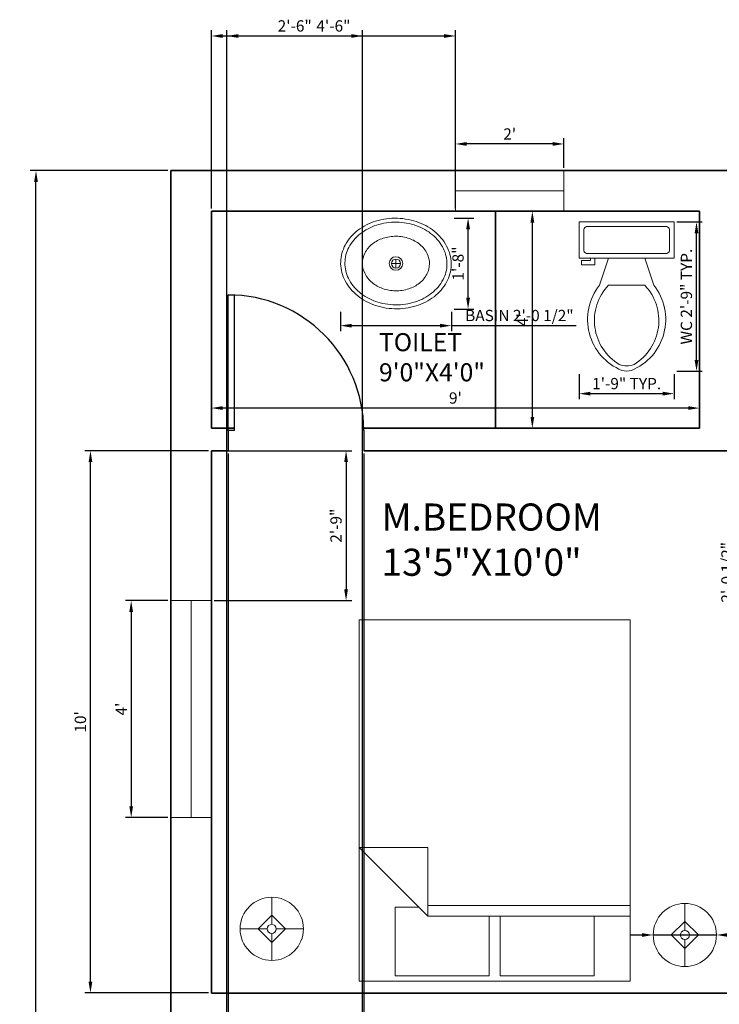
# Model space of a CAD drawing. Units: inches. Extents: x 3889 to 4254, y 3310 to 3958.
# Tile 5 of 6: x 3891 to 4046, y 3738 to 3956. Entities that reach past the tile are written whole.
import ezdxf

# ---------------------------------------------------------------- set-up
doc = ezdxf.new("R2010")
doc.units = ezdxf.units.IN
for name, color, linetype, lineweight in [('A-AREA-IDEN', 11, 'Continuous', 18), ('A-FLOR-FIXT', 130, 'Continuous', 18), ('A-WALL', 7, 'Continuous', 35), ('DIM', 81, 'Continuous', 18), ('DOOR', 1, 'Continuous', 25), ('FURNITURES', 130, 'Continuous', 18), ('WINDOW', 3, 'Continuous', 18)]:
    doc.layers.add(name, color=color, linetype=linetype, lineweight=lineweight)
doc.styles.get("Standard").update_dxf_attribs({"font": 'arial.ttf'})
doc.dimstyles.new('ISO-25', dxfattribs={"dimtxt": 2.5, "dimasz": 2.5, "dimexe": 1.25, "dimexo": 0.625, "dimtad": 1, "dimlunit": 3, "dimtxsty": 'Standard', "dimcen": 2.5, "dimadec": 0, "dimazin": 0, "dimtfac": 1, "dimtmove": 0, "dimatfit": 3, "dimfxl": 1, "dimarcsym": 0})

# ---------------------------------------------------------------- blocks, each defined once
blk = doc.blocks.new('*U4')
for p, q in [((0, 0), (0, -6)), ((40, 0), (40, -6))]:
    blk.add_line(p, q)
blk.add_lwpolyline([(0, 0), (0, 40), (1.75, 40), (1.75, 0)], close=True)
blk.add_arc((0, 0), 40, 0, 90)
blk = doc.blocks.new('Sink - Oval top')
for p, q in [((-1, 0), (1, 0)), ((0, 1), (0, -1))]:
    blk.add_line(p, q)
for points in [[(-12.23, 0.39, 0.117634), (-11.46, -3.36, 0.104469), (-8.88, -6.8, 0.090016), (-5.08, -9.07, 0.08192), (-0.32, -10.02, 0.08192), (4.49, -9.38, 0.090016), (8.42, -7.36, 0.104469), (11.22, -4.09, 0.117634), (12.23, -0.39, 0.117634), (11.46, 3.36, 0.104469), (8.88, 6.8, 0.090016), (5.08, 9.07, 0.08192), (0.32, 10.02, 0.08192), (-4.49, 9.38, 0.090016), (-8.42, 7.36, 0.104469), (-11.22, 4.09, 0.117634)], [(-11.29, 0.16, 0.118622), (-10.52, -3.25, 0.104678), (-8.07, -6.36, 0.089562), (-4.54, -8.37, 0.081185), (-0.13, -9.15, 0.081185), (4.3, -8.49, 0.089562), (7.89, -6.58, 0.104678), (10.42, -3.55, 0.118622), (11.29, -0.16, 0.118622), (10.52, 3.25, 0.104678), (8.07, 6.36, 0.089562), (4.54, 8.37, 0.081185), (0.13, 9.15, 0.081185), (-4.3, 8.49, 0.089562), (-7.89, 6.58, 0.104678), (-10.42, 3.55, 0.118622)], [(-7.42, 0.08, 0.118283), (-6.91, -2.17, 0.104607), (-5.29, -4.21, 0.089718), (-2.97, -5.53, 0.081436), (-0.07, -6.04, 0.081436), (2.84, -5.59, 0.089718), (5.2, -4.33, 0.104607), (6.86, -2.32, 0.118283), (7.42, -0.08, 0.118283), (6.91, 2.17, 0.104607), (5.29, 4.21, 0.089718), (2.97, 5.53, 0.081436), (0.07, 6.04, 0.081436), (-2.84, 5.59, 0.089718), (-5.2, 4.33, 0.104607), (-6.86, 2.32, 0.118283)]]:
    blk.add_lwpolyline(points, format="xyb", close=True)
for radius in [1.5, 1]:
    blk.add_circle((0, 0), radius)
blk = doc.blocks.new('Bed - Queen')
for p, q in [((0, -80.00003), (0, 0)), ((0, 0), (59.99999, 0)), ((59.99999, 0), (59.99999, -80.00003)), ((7.99999, -1.2), (28.79998, -1.2)), ((7.99999, -14.4), (7.99999, -1.2)), ((28.79998, -1.2), (28.79998, -14.4)), ((31.19999, -1.2), (51.99999, -1.2)), ((31.19999, -14.4), (31.19999, -1.2)), ((51.99999, -1.2), (51.99999, -16.4)), ((0, -14.4), (44.8, -14.4)), ((59.99999, -29.6), (44.8, -14.4)), ((44.8, -14.4), (44.8, -29.6)), ((44.8, -16.8), (0, -16.8)), ((51.99999, -16.4), (46.79936, -16.4)), ((44.8, -29.6), (59.99999, -29.6)), ((59.99999, -80.00003), (0, -80.00003))]:
    blk.add_line(p, q)
blk = doc.blocks.new('Lamp - Table')
for p, q in [((0, 7), (0, 1)), ((0, 3), (-3, 0)), ((3, 0), (0, 3)), ((-1, 0), (-7, 0)), ((-3, 0), (0, -3)), ((0, -3), (3, 0)), ((1, 0), (7, 0)), ((0, -1), (0, -7))]:
    blk.add_line(p, q)
for radius in [7, 1]:
    blk.add_circle((0, 0), radius)
blk = doc.blocks.new('Toilet - top')
for p, q in [((9.5, -6), (9.5, -2)), ((-10, -8.5), (-8, -8.5)), ((-10, -9.5), (-10, -8.5)), ((-8, -8.5), (-8, -8)), ((-7, -8), (-7, -9.5)), ((-4, -8), (-6, -14)), ((4, -8), (6, -14)), ((-7, -9.5), (-10, -9.5)), ((4, -14), (-4, -14))]:
    blk.add_line(p, q)
blk.add_lwpolyline([(10.5, -8), (10.5, 0), (-10.5, 0), (-10.5, -8)], close=True)
for points in [[(-9.5, -2), (-9.5, -6)], [(8.5, -1), (-8.5, -1)], [(-8.5, -7), (8.5, -7)]]:
    blk.add_lwpolyline(points)
for centre, radius, start, end in [((-8.62, -1.88), 0.884, 81.8699, 188.1301), ((8.62, -1.88), 0.884, 351.8699, 98.1301), ((-8.62, -6.12), 0.884, 171.8699, 278.1301), ((8.62, -6.12), 0.884, 261.8699, 8.1301), ((3.52, -21.58), 12.17, 141.4691, 247.9714), ((4.2, -21.82), 11.33, 136.3677, 238.9468), ((-3.52, -21.58), 12.17, 292.0284, 38.5307), ((-4.2, -21.82), 11.33, 301.053, 43.6321), ((0, -27.88), 4, 245.7318, 294.2682), ((0, -29), 4, 254.8605, 285.1395)]:
    blk.add_arc(centre, radius, start, end)
blk = doc.blocks.new('*D21')
at = {"layer": 'Defpoints', "color": 0, "transparency": 16777216}
for p in [(3924.84, 3826.95), (3916.1, 3778.95), (3924.84, 3778.95)]:
    blk.add_point(p, dxfattribs=at)
at = {"layer": 'DIM', "color": 0, "lineweight": -2, "transparency": 16777216}
for p, q in [((3924.22, 3826.95), (3914.85, 3826.95)), ((3916.1, 3824.45), (3916.1, 3781.45)), ((3924.22, 3778.95), (3914.85, 3778.95))]:
    blk.add_line(p, q, dxfattribs=at)
at = {"layer": 'DIM', "color": 0, "transparency": 16777216}
for points in [[(3915.69, 3824.45), (3916.52, 3824.45), (3916.1, 3826.95)], [(3915.69, 3781.45), (3916.52, 3781.45), (3916.1, 3778.95)]]:
    blk.add_solid(points, dxfattribs=at)
at = {"layer": 'DIM', "color": 0, "transparency": 16777216, "insert": (3914.23, 3802.95), "char_height": 2.5, "attachment_point": 5, "rotation": 90}
blk.add_mtext("4'", dxfattribs=at)
blk = doc.blocks.new('*D33')
at = {"layer": 'Defpoints', "color": 0, "transparency": 16777216}
for p in [(3996.71, 3913.11), (4004.86, 3913.11), (3996.71, 3865.11)]:
    blk.add_point(p, dxfattribs=at)
at = {"layer": 'DIM', "color": 0, "lineweight": -2, "transparency": 16777216}
for p, q in [((3997.33, 3913.11), (4006.11, 3913.11)), ((4004.86, 3867.61), (4004.86, 3910.61)), ((3997.33, 3865.11), (4006.11, 3865.11))]:
    blk.add_line(p, q, dxfattribs=at)
at = {"layer": 'DIM', "color": 0, "transparency": 16777216}
for points in [[(4004.44, 3910.61), (4005.28, 3910.61), (4004.86, 3913.11)], [(4004.44, 3867.61), (4005.28, 3867.61), (4004.86, 3865.11)]]:
    blk.add_solid(points, dxfattribs=at)
at = {"layer": 'DIM', "color": 0, "transparency": 16777216, "insert": (4002.99, 3889.11), "char_height": 2.5, "attachment_point": 5, "rotation": 90}
blk.add_mtext("4'", dxfattribs=at)
blk = doc.blocks.new('*D34')
at = {"layer": 'Defpoints', "color": 0, "transparency": 16777216}
for p in [(3933.84, 3869.56), (3933.84, 3865.11), (4041.84, 3865.11)]:
    blk.add_point(p, dxfattribs=at)
at = {"layer": 'DIM', "color": 0, "lineweight": -2, "transparency": 16777216}
for p, q in [((3933.84, 3865.73), (3933.84, 3870.81)), ((4041.84, 3865.73), (4041.84, 3870.81)), ((4039.34, 3869.56), (3936.34, 3869.56))]:
    blk.add_line(p, q, dxfattribs=at)
at = {"layer": 'DIM', "color": 0, "transparency": 16777216}
for points in [[(3936.34, 3869.98), (3936.34, 3869.15), (3933.84, 3869.56)], [(4039.34, 3869.98), (4039.34, 3869.15), (4041.84, 3869.56)]]:
    blk.add_solid(points, dxfattribs=at)
at = {"layer": 'DIM', "color": 0, "transparency": 16777216, "insert": (3987.84, 3871.46), "char_height": 2.5, "attachment_point": 5}
blk.add_mtext("9'", dxfattribs=at)
blk = doc.blocks.new('*D35')
at = {"layer": 'Defpoints', "color": 0, "transparency": 16777216}
for p in [(3987.84, 3928.01), (3987.84, 3922.11), (4011.84, 3922.11)]:
    blk.add_point(p, dxfattribs=at)
at = {"layer": 'DIM', "color": 0, "lineweight": -2, "transparency": 16777216}
for p, q in [((3987.84, 3922.73), (3987.84, 3929.26)), ((4011.84, 3922.73), (4011.84, 3929.26)), ((4009.34, 3928.01), (3990.34, 3928.01))]:
    blk.add_line(p, q, dxfattribs=at)
at = {"layer": 'DIM', "color": 0, "transparency": 16777216}
for points in [[(3990.34, 3928.43), (3990.34, 3927.6), (3987.84, 3928.01)], [(4009.34, 3928.43), (4009.34, 3927.6), (4011.84, 3928.01)]]:
    blk.add_solid(points, dxfattribs=at)
at = {"layer": 'DIM', "color": 0, "transparency": 16777216, "insert": (3999.84, 3929.89), "char_height": 2.5, "attachment_point": 5}
blk.add_mtext("2'", dxfattribs=at)
blk = doc.blocks.new('*D38')
at = {"layer": 'Defpoints', "color": 0, "transparency": 16777216}
for p in [(3907.09, 3860.11), (3933.84, 3860.11), (3933.84, 3740.11)]:
    blk.add_point(p, dxfattribs=at)
at = {"layer": 'DIM', "color": 0, "lineweight": -2, "transparency": 16777216}
for p, q in [((3933.22, 3860.11), (3905.84, 3860.11)), ((3907.09, 3742.61), (3907.09, 3857.61)), ((3933.22, 3740.11), (3905.84, 3740.11))]:
    blk.add_line(p, q, dxfattribs=at)
at = {"layer": 'DIM', "color": 0, "transparency": 16777216}
for points in [[(3906.68, 3857.61), (3907.51, 3857.61), (3907.09, 3860.11)], [(3906.68, 3742.61), (3907.51, 3742.61), (3907.09, 3740.11)]]:
    blk.add_solid(points, dxfattribs=at)
at = {"layer": 'DIM', "color": 0, "transparency": 16777216, "insert": (3905.19, 3800.11), "char_height": 2.5, "attachment_point": 5, "rotation": 90}
blk.add_mtext("10'", dxfattribs=at)
blk = doc.blocks.new('WIN-48x9')
blk.add_line((4.5, 48), (4.5, 0))
blk.add_lwpolyline([(0, 48), (9, 48), (9, 0), (0, 0)], close=True)
blk = doc.blocks.new('WIN-24x9')
blk.add_line((24, 4.5), (0, 4.5))
blk.add_lwpolyline([(24, 9), (24, 0), (0, 0), (0, 9)], close=True)
blk = doc.blocks.new('*D45')
at = {"layer": 'Defpoints', "color": 0, "transparency": 16777216}
for p in [(4036.22, 3910.75), (4041.18, 3910.75), (4036.22, 3877.71)]:
    blk.add_point(p, dxfattribs=at)
at = {"layer": 'DIM', "color": 0, "lineweight": -2, "transparency": 16777216}
for p, q in [((4036.84, 3910.75), (4042.43, 3910.75)), ((4041.18, 3880.21), (4041.18, 3908.25)), ((4036.84, 3877.71), (4042.43, 3877.71))]:
    blk.add_line(p, q, dxfattribs=at)
at = {"layer": 'DIM', "color": 0, "transparency": 16777216}
for points in [[(4040.76, 3908.25), (4041.59, 3908.25), (4041.18, 3910.75)], [(4040.76, 3880.21), (4041.59, 3880.21), (4041.18, 3877.71)]]:
    blk.add_solid(points, dxfattribs=at)
at = {"layer": 'DIM', "color": 0, "transparency": 16777216, "insert": (4039.26, 3894.23), "char_height": 2.5, "attachment_point": 5, "rotation": 90}
blk.add_mtext('WC 2\'-9" TYP.', dxfattribs=at)
blk = doc.blocks.new('*D46')
at = {"layer": 'Defpoints', "color": 0, "transparency": 16777216}
for p in [(4015.22, 3877.71), (4036.22, 3877.71), (4036.22, 3872.75)]:
    blk.add_point(p, dxfattribs=at)
at = {"layer": 'DIM', "color": 0, "lineweight": -2, "transparency": 16777216}
for p, q in [((4015.22, 3877.08), (4015.22, 3871.5)), ((4036.22, 3877.08), (4036.22, 3871.5)), ((4017.72, 3872.75), (4033.72, 3872.75))]:
    blk.add_line(p, q, dxfattribs=at)
at = {"layer": 'DIM', "color": 0, "transparency": 16777216}
for points in [[(4017.72, 3873.17), (4017.72, 3872.33), (4015.22, 3872.75)], [(4033.72, 3873.17), (4033.72, 3872.33), (4036.22, 3872.75)]]:
    blk.add_solid(points, dxfattribs=at)
at = {"layer": 'DIM', "color": 0, "transparency": 16777216, "insert": (4025.72, 3874.65), "char_height": 2.5, "attachment_point": 5}
blk.add_mtext('1\'-9" TYP.', dxfattribs=at)
blk = doc.blocks.new('*D47')
at = {"layer": 'Defpoints', "color": 0, "transparency": 16777216}
for p in [(3962.4, 3891.48), (3986.96, 3891.48), (3986.96, 3887.8)]:
    blk.add_point(p, dxfattribs=at)
at = {"layer": 'DIM', "color": 0, "lineweight": -2, "transparency": 16777216}
for p, q in [((3962.4, 3890.86), (3962.4, 3886.55)), ((3986.96, 3890.86), (3986.96, 3886.55)), ((3964.9, 3887.8), (3984.46, 3887.8)), ((3986.96, 3887.8), (4014.52, 3887.8))]:
    blk.add_line(p, q, dxfattribs=at)
at = {"layer": 'DIM', "color": 0, "transparency": 16777216}
for points in [[(3964.9, 3888.21), (3964.9, 3887.38), (3962.4, 3887.8)], [(3984.46, 3888.21), (3984.46, 3887.38), (3986.96, 3887.8)]]:
    blk.add_solid(points, dxfattribs=at)
at = {"layer": 'DIM', "color": 0, "transparency": 16777216, "insert": (4001.99, 3889.72), "char_height": 2.5, "attachment_point": 5}
blk.add_mtext('BASIN 2\'-0 1/2"', dxfattribs=at)
blk = doc.blocks.new('*D48')
at = {"layer": 'Defpoints', "color": 0, "transparency": 16777216}
for p in [(3986.96, 3911.62), (3990.64, 3911.62), (3986.96, 3891.48)]:
    blk.add_point(p, dxfattribs=at)
at = {"layer": 'DIM', "color": 0, "lineweight": -2, "transparency": 16777216}
for p, q in [((3987.58, 3911.62), (3991.89, 3911.62)), ((3990.64, 3893.98), (3990.64, 3909.12)), ((3987.58, 3891.48), (3991.89, 3891.48))]:
    blk.add_line(p, q, dxfattribs=at)
at = {"layer": 'DIM', "color": 0, "transparency": 16777216}
for points in [[(3990.22, 3909.12), (3991.06, 3909.12), (3990.64, 3911.62)], [(3990.22, 3893.98), (3991.06, 3893.98), (3990.64, 3891.48)]]:
    blk.add_solid(points, dxfattribs=at)
at = {"layer": 'DIM', "color": 0, "transparency": 16777216, "insert": (3988.74, 3901.55), "char_height": 2.5, "attachment_point": 5, "rotation": 90}
blk.add_mtext('1\'-8"', dxfattribs=at)
blk = doc.blocks.new('*D66')
at = {"layer": 'Defpoints', "color": 0, "transparency": 16777216}
for p in [(4050.16, 3845.42), (4054.21, 3845.42), (4054.21, 3820.99)]:
    blk.add_point(p, dxfattribs=at)
at = {"layer": 'DIM', "color": 0, "lineweight": -2, "transparency": 16777216}
for p, q in [((4053.58, 3845.42), (4048.91, 3845.42)), ((4050.16, 3823.49), (4050.16, 3842.92)), ((4053.58, 3820.99), (4048.91, 3820.99))]:
    blk.add_line(p, q, dxfattribs=at)
at = {"layer": 'DIM', "color": 0, "transparency": 16777216}
for points in [[(4049.74, 3842.92), (4050.57, 3842.92), (4050.16, 3845.42)], [(4049.74, 3823.49), (4050.57, 3823.49), (4050.16, 3820.99)]]:
    blk.add_solid(points, dxfattribs=at)
at = {"layer": 'DIM', "color": 0, "transparency": 16777216, "insert": (4048.24, 3833.21), "char_height": 2.5, "attachment_point": 5, "rotation": 90}
blk.add_mtext('2\'-0 1/2"', dxfattribs=at)
blk = doc.blocks.new('*D72')
at = {"layer": 'Defpoints', "color": 0, "transparency": 16777216}
for p in [(3933.84, 3860.11), (3933.84, 3826.95), (3963.64, 3826.95)]:
    blk.add_point(p, dxfattribs=at)
at = {"layer": 'DIM', "color": 0, "lineweight": -2, "transparency": 16777216}
for p, q in [((3934.47, 3860.11), (3964.89, 3860.11)), ((3963.64, 3857.61), (3963.64, 3829.45)), ((3934.47, 3826.95), (3964.89, 3826.95))]:
    blk.add_line(p, q, dxfattribs=at)
at = {"layer": 'DIM', "color": 0, "transparency": 16777216}
for points in [[(3963.23, 3857.61), (3964.06, 3857.61), (3963.64, 3860.11)], [(3963.23, 3829.45), (3964.06, 3829.45), (3963.64, 3826.95)]]:
    blk.add_solid(points, dxfattribs=at)
at = {"layer": 'DIM', "color": 0, "transparency": 16777216, "insert": (3961.74, 3843.53), "char_height": 2.5, "attachment_point": 5, "rotation": 90}
blk.add_mtext('2\'-9"', dxfattribs=at)
blk = doc.blocks.new('*D75')
at = {"layer": 'Defpoints', "color": 0, "transparency": 16777216}
for p in [(3987.84, 3951.91), (3933.84, 3913.11), (3987.84, 3913.11)]:
    blk.add_point(p, dxfattribs=at)
at = {"layer": 'DIM', "color": 0, "lineweight": -2, "transparency": 16777216}
for p, q in [((3933.84, 3913.73), (3933.84, 3953.16)), ((3987.84, 3913.73), (3987.84, 3953.16)), ((3936.34, 3951.91), (3985.34, 3951.91))]:
    blk.add_line(p, q, dxfattribs=at)
at = {"layer": 'DIM', "color": 0, "transparency": 16777216}
for points in [[(3936.34, 3952.32), (3936.34, 3951.49), (3933.84, 3951.91)], [(3985.34, 3952.32), (3985.34, 3951.49), (3987.84, 3951.91)]]:
    blk.add_solid(points, dxfattribs=at)
at = {"layer": 'DIM', "color": 0, "transparency": 16777216, "insert": (3960.84, 3953.81), "char_height": 2.5, "attachment_point": 5}
blk.add_mtext('4\'-6"', dxfattribs=at)
blk = doc.blocks.new('*D92')
at = {"layer": 'Defpoints', "color": 0, "transparency": 16777216}
for p in [(3937.55, 3860.11), (3967.55, 3860.11), (3967.55, 3312.31)]:
    blk.add_point(p, dxfattribs=at)
at = {"layer": 'DIM', "color": 0, "lineweight": -2, "transparency": 16777216}
for p, q in [((3937.55, 3859.48), (3937.55, 3311.06)), ((3967.55, 3859.48), (3967.55, 3311.06)), ((3940.05, 3312.31), (3965.05, 3312.31))]:
    blk.add_line(p, q, dxfattribs=at)
at = {"layer": 'DIM', "color": 0, "transparency": 16777216}
for points in [[(3940.05, 3312.72), (3940.05, 3311.89), (3937.55, 3312.31)], [(3965.05, 3312.72), (3965.05, 3311.89), (3967.55, 3312.31)]]:
    blk.add_solid(points, dxfattribs=at)
at = {"layer": 'DIM', "color": 0, "transparency": 16777216, "insert": (3952.55, 3314.21), "char_height": 2.5, "attachment_point": 5}
blk.add_mtext('2\'-6"', dxfattribs=at)
blk = doc.blocks.new('*D93')
at = {"layer": 'Defpoints', "color": 0, "transparency": 16777216}
for p in [(3967.28, 3951.91), (3937.28, 3615.11), (3967.28, 3615.11)]:
    blk.add_point(p, dxfattribs=at)
at = {"layer": 'DIM', "color": 0, "lineweight": -2, "transparency": 16777216}
for p, q in [((3937.28, 3615.73), (3937.28, 3953.16)), ((3967.28, 3615.73), (3967.28, 3953.16)), ((3939.78, 3951.91), (3964.78, 3951.91))]:
    blk.add_line(p, q, dxfattribs=at)
at = {"layer": 'DIM', "color": 0, "transparency": 16777216}
for points in [[(3939.78, 3952.32), (3939.78, 3951.49), (3937.28, 3951.91)], [(3964.78, 3952.32), (3964.78, 3951.49), (3967.28, 3951.91)]]:
    blk.add_solid(points, dxfattribs=at)
at = {"layer": 'DIM', "color": 0, "transparency": 16777216, "insert": (3952.28, 3953.81), "char_height": 2.5, "attachment_point": 5}
blk.add_mtext('2\'-6"', dxfattribs=at)
blk = doc.blocks.new('*D97')
at = {"layer": 'Defpoints', "color": 0, "transparency": 16777216}
for p in [(3895.04, 3922.11), (3924.84, 3922.11), (3924.84, 3342.11)]:
    blk.add_point(p, dxfattribs=at)
at = {"layer": 'DIM', "color": 0, "lineweight": -2, "transparency": 16777216}
for p, q in [((3924.22, 3922.11), (3893.79, 3922.11)), ((3895.04, 3344.61), (3895.04, 3919.61)), ((3924.22, 3342.11), (3893.79, 3342.11))]:
    blk.add_line(p, q, dxfattribs=at)
at = {"layer": 'DIM', "color": 0, "transparency": 16777216}
for points in [[(3894.63, 3919.61), (3895.46, 3919.61), (3895.04, 3922.11)], [(3894.63, 3344.61), (3895.46, 3344.61), (3895.04, 3342.11)]]:
    blk.add_solid(points, dxfattribs=at)
at = {"layer": 'DIM', "color": 0, "transparency": 16777216, "insert": (3893.14, 3632.11), "char_height": 2.5, "attachment_point": 5, "rotation": 90}
blk.add_mtext('48\'-4"', dxfattribs=at)
blk = doc.blocks.new('*D98')
at = {"layer": 'Defpoints', "color": 0, "transparency": 16777216}
for p in [(4031.6, 3752.95), (4045.6, 3752.95)]:
    blk.add_point(p, dxfattribs=at)
at = {"layer": 'DIM', "color": 0, "lineweight": -2, "transparency": 16777216}
for p, q in [((4029.1, 3752.94), (4026.6, 3752.94)), ((4031.6, 3752.95), (4045.6, 3752.95)), ((4066.45, 3752.95), (4048.1, 3752.95))]:
    blk.add_line(p, q, dxfattribs=at)
at = {"layer": 'DIM', "color": 0, "transparency": 16777216}
for points in [[(4029.1, 3753.36), (4029.1, 3752.53), (4031.6, 3752.95)], [(4048.1, 3753.37), (4048.1, 3752.53), (4045.6, 3752.95)]]:
    blk.add_solid(points, dxfattribs=at)
at = {"layer": 'DIM', "color": 0, "transparency": 16777216, "insert": (4058.52, 3754.92), "char_height": 2.5, "attachment_point": 5, "rotation": 0.0136}
blk.add_mtext('3X ∅1\'-2"', dxfattribs=at)

msp = doc.modelspace()

# ---------------------------------------------------------------- linework, layer by layer
at = {"layer": 'A-WALL'}
for p, q in [((3924.843, 3342.107), (3924.843, 3922.107)), ((3924.843, 3922.107), (4222.843, 3922.107)), ((3933.843, 3913.107), (4041.843, 3913.107)), ((3933.843, 3865.107), (3933.843, 3913.107)), ((3996.71, 3913.107), (3996.71, 3865.107)), ((4041.843, 3865.107), (4041.843, 3913.107)), ((3933.843, 3865.107), (3938.858, 3865.107)), ((3967.541, 3865.107), (4041.843, 3865.107)), ((3933.843, 3860.107), (3937.546, 3860.107)), ((3933.843, 3740.107), (3933.843, 3860.107)), ((3967.546, 3860.107), (4098.843, 3860.107)), ((3933.843, 3740.107), (4067.084, 3740.107))]:
    msp.add_line(p, q, dxfattribs=at)

# ---------------------------------------------------------------- block references
at = {"layer": 'A-FLOR-FIXT'}
for name, p in [('Sink - Oval top', (3974.68, 3901.549)), ('Toilet - top', (4025.719, 3910.754))]:
    msp.add_blockref(name, p, dxfattribs=at)
at = {"layer": 'DOOR', "xscale": 0.75, "yscale": 0.75, "zscale": 0.75}
msp.add_blockref('*U4', (3937.546, 3864.607), dxfattribs=at)
at = {"layer": 'FURNITURES', "rotation": 180}
msp.add_blockref('Bed - Queen', (4026.527, 3742.707), dxfattribs=at)
at = {"layer": 'FURNITURES'}
for p in [(3947.211, 3754.309), (4038.597, 3752.947)]:
    msp.add_blockref('Lamp - Table', p, dxfattribs=at)
at = {"layer": 'WINDOW'}
for name, p in [('WIN-24x9', (3987.843, 3913.107)), ('WIN-48x9', (3924.843, 3778.948))]:
    msp.add_blockref(name, p, dxfattribs=at)

# ---------------------------------------------------------------- texts
at = {"layer": 'A-AREA-IDEN', "attachment_point": 1}
for s, insert, char_height in [('TOILET\\P9\'0"X4\'0"', (3970.93, 3886.142), 4), ('M.BEDROOM\\P13\'5"X10\'0"', (3971.496, 3848.442), 6)]:
    msp.add_mtext_dynamic_manual_height_columns(s, width=76.4548, gutter_width=12.5, heights=[0], dxfattribs=dict(at, insert=insert, char_height=char_height))

# ---------------------------------------------------------------- dimensions: what is measured, and where the dimension line sits
at = {"layer": 'DIM'}
for base, p1, p2, override, picture, middle in [((3987.843, 3951.907), (3933.843, 3913.107), (3987.843, 3913.107), {"dimdec": 1, "dimlfac": 1, "dimrnd": 0, "dimzin": 1, "dimdsep": 46, "dimlunit": 4, "dimfrac": 2}, '*D75', (3960.843, 3953.808)), ((3967.284, 3951.907), (3937.284, 3615.107), (3967.284, 3615.107), {"dimdec": 1, "dimlfac": 1, "dimrnd": 0, "dimzin": 1, "dimdsep": 46, "dimlunit": 4, "dimfrac": 2}, '*D93', (3952.284, 3953.808)), ((3987.843, 3928.013), (4011.843, 3922.107), (3987.843, 3922.107), {"dimclrd": 0, "dimclre": 0, "dimclrt": 0}, '*D35', (3999.843, 3929.893)), ((3933.843, 3869.563), (4041.843, 3865.107), (3933.843, 3865.107), {"dimclrd": 0, "dimclre": 0, "dimclrt": 0}, '*D34', (3987.843, 3871.465)), ((3967.546, 3312.307), (3937.546, 3860.107), (3967.546, 3860.107), {"dimdec": 1, "dimlfac": 1, "dimrnd": 0, "dimzin": 1, "dimdsep": 46, "dimlunit": 4, "dimfrac": 2}, '*D92', (3952.546, 3314.208))]:
    dim = msp.add_linear_dim(base=base, p1=p1, p2=p2, dimstyle='ISO-25', override=override, dxfattribs=at)
    dim.commit()
    dim.dimension.update_dxf_attribs({"geometry": picture, "text_midpoint": middle})
for base, p1, p2, angle, override, picture, middle in [((3895.043, 3922.107), (3924.843, 3342.107), (3924.843, 3922.107), 90, {"dimdec": 1, "dimlfac": 1, "dimrnd": 0, "dimzin": 1, "dimdsep": 46, "dimlunit": 4, "dimfrac": 2}, '*D97', (3893.141, 3632.107)), ((3990.638, 3911.617), (3986.956, 3891.481), (3986.956, 3911.617), 90, {"dimdec": 1, "dimlfac": 1, "dimrnd": 0, "dimzin": 1, "dimdsep": 46, "dimlunit": 4, "dimfrac": 2}, '*D48', (3988.737, 3901.549)), ((4004.861, 3913.107), (3996.71, 3865.107), (3996.71, 3913.107), 90, {"dimclrd": 0, "dimclre": 0, "dimclrt": 0}, '*D33', (4002.986, 3889.107)), ((3907.093, 3860.107), (3933.843, 3740.107), (3933.843, 3860.107), 90, {"dimclrd": 0, "dimclre": 0, "dimclrt": 0}, '*D38', (3905.191, 3800.107)), ((3963.643, 3826.948), (3933.843, 3860.107), (3933.843, 3826.948), 270, {"dimdec": 1, "dimlfac": 1, "dimrnd": 0, "dimzin": 1, "dimdsep": 46, "dimlunit": 4, "dimfrac": 2}, '*D72', (3961.741, 3843.527)), ((4050.156, 3845.423), (4054.206, 3820.988), (4054.206, 3845.423), 90, {"dimdec": 1, "dimlfac": 1, "dimrnd": 0, "dimzin": 1, "dimdsep": 46, "dimlunit": 4, "dimfrac": 2}, '*D66', (4048.239, 3833.205)), ((3916.102, 3778.948), (3924.843, 3826.948), (3924.843, 3778.948), 90, {"dimclrd": 0, "dimclre": 0, "dimclrt": 0}, '*D21', (3914.227, 3802.948))]:
    dim = msp.add_linear_dim(base=base, p1=p1, p2=p2, angle=angle, dimstyle='ISO-25', override=override, dxfattribs=at)
    dim.commit()
    dim.dimension.update_dxf_attribs({"geometry": picture, "text_midpoint": middle})
dim = msp.add_linear_dim(base=(4041.176, 3910.754), p1=(4036.219, 3877.708), p2=(4036.219, 3910.754), angle=90, text='WC <> TYP.', dimstyle='ISO-25', override={"dimdec": 1, "dimlfac": 1, "dimrnd": 0, "dimzin": 1, "dimdsep": 46, "dimlunit": 4, "dimfrac": 2}, dxfattribs=at)
dim.commit()
dim.dimension.update_dxf_attribs({"geometry": '*D45', "text_midpoint": (4039.259, 3894.231)})
for base, p1, p2, text, picture, middle in [((3986.956, 3887.798), (3962.405, 3891.481), (3986.956, 3891.481), 'BASIN <>', '*D47', (4001.987, 3889.716)), ((4036.219, 3872.751), (4015.219, 3877.708), (4036.219, 3877.708), '<> TYP.', '*D46', (4025.719, 3874.653))]:
    dim = msp.add_linear_dim(base=base, p1=p1, p2=p2, text=text, dimstyle='ISO-25', override={"dimdec": 1, "dimlfac": 1, "dimrnd": 0, "dimzin": 1, "dimdsep": 46, "dimlunit": 4, "dimfrac": 2}, dxfattribs=at)
    dim.commit()
    dim.dimension.update_dxf_attribs({"geometry": picture, "text_midpoint": middle})
dim = msp.add_diameter_dim_2p(p1=(4031.597, 3752.945), p2=(4045.597, 3752.948), text='3X <>', dimstyle='ISO-25', override={"dimdec": 1, "dimlfac": 1, "dimrnd": 0, "dimzin": 1, "dimdsep": 46, "dimlunit": 4, "dimfrac": 2}, dxfattribs=at)
dim.commit()
dim.dimension.update_dxf_attribs({"geometry": '*D98', "text_midpoint": (4058.524, 3752.951), "dimtype": 163})

doc.saveas('drawing.dxf')
